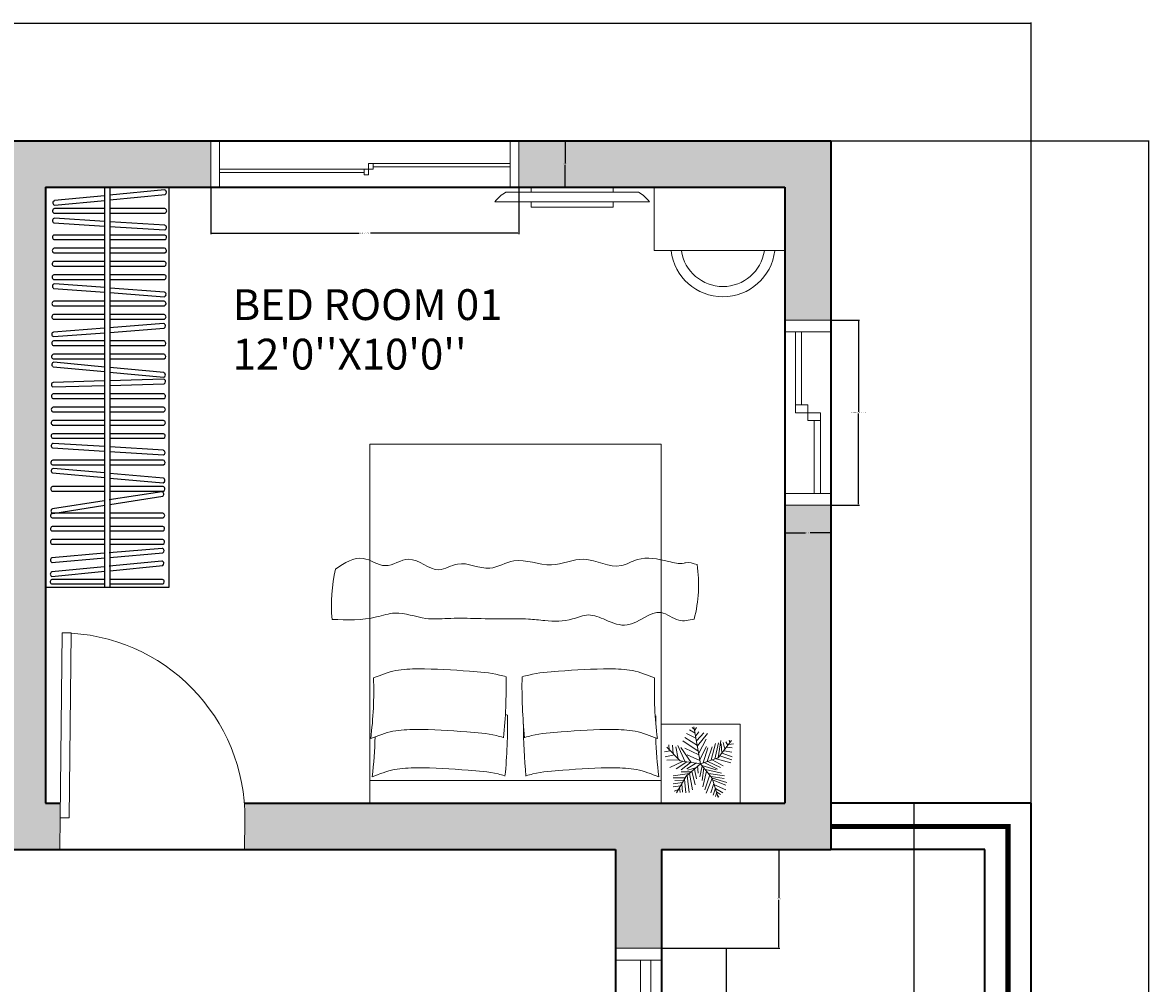
# Model space of a CAD drawing. Units: inches. Extents: x 1789 to 2841, y 3180 to 3702.
# Tile 14 of 14: x 2606 to 2825, y 3491 to 3678. Entities that reach past the tile are written whole.
import ezdxf

# ---------------------------------------------------------------- set-up
doc = ezdxf.new("R2010")
doc.units = ezdxf.units.IN
doc.header["$MEASUREMENT"] = 0
for name, color, linetype, lineweight in [('A-ANNO-DIMS', 2, 'Continuous', 18), ('A-AREA-IDEN', 7, 'Continuous', 18), ('A-EQPM', 8, 'Continuous', 18), ('A-FLOR-CASE', 34, 'Continuous', 25), ('A-FLOR-HRAL', 40, 'Continuous', 18), ('A-WALL', 40, 'Continuous', 35), ('A-WALL-PATT', 252, 'Continuous', 13), ('DORS', 70, 'Continuous', 18), ('FURNITURE', 34, 'Continuous', 18), ('WINDOWS', 130, 'Continuous', 18)]:
    doc.layers.add(name, color=color, linetype=linetype, lineweight=lineweight)
doc.styles.get("Standard").update_dxf_attribs({"font": 'arial.ttf'})
doc.dimstyles.get("Standard").update_dxf_attribs({"dimtxt": 0.18, "dimasz": 0.18, "dimexe": 0.18, "dimexo": 0.0625, "dimgap": 0.09, "dimtad": 0, "dimtih": 1, "dimtoh": 1, "dimdec": 0, "dimzin": 0, "dimdsep": 46, "dimlunit": 3, "dimtxsty": 'Standard', "dimcen": 0.09, "dimadec": 0, "dimazin": 0, "dimtfac": 1, "dimtdec": 0, "dimtofl": 0, "dimtmove": 0, "dimatfit": 3, "dimfxl": 1, "dimtolj": 1, "dimtzin": 0, "dimarcsym": 0})

# ---------------------------------------------------------------- blocks, each defined once
blk = doc.blocks.new('HYJ')
for p, q in [((2206.12, 3649.67), (2234.3, 3649.67)), ((2206.12, 3649), (2234.3, 3649)), ((2236.02, 3650.77), (2262.74, 3650.77)), ((2236.02, 3650.11), (2262.74, 3650.11))]:
    blk.add_line(p, q)
for points in [[(2204.43, 3646.16), (2264.43, 3646.16), (2264.43, 3655.16), (2204.43, 3655.16)], [(2204.43, 3655.16), (2206.12, 3655.16), (2206.12, 3646.16), (2204.43, 3646.16)], [(2264.43, 3655.16), (2262.74, 3655.16), (2262.74, 3646.16), (2264.43, 3646.16)], [(2234.3, 3649.67), (2235.16, 3649.67), (2235.16, 3648.56), (2234.3, 3648.56)], [(2235.16, 3650.77), (2236.02, 3650.77), (2236.02, 3649.67), (2235.16, 3649.67)]]:
    blk.add_lwpolyline(points, close=True)
blk = doc.blocks.new('KIK')
for p, q in [((2336.3, 3607.04), (2336.3, 3621.23)), ((2337.52, 3607.04), (2337.52, 3621.23)), ((2339.95, 3603.98), (2339.95, 3589.79)), ((2341.17, 3603.98), (2341.17, 3589.79))]:
    blk.add_line(p, q)
for points in [[(2343.23, 3623.51), (2343.23, 3587.51), (2334.23, 3587.51), (2334.23, 3623.51)], [(2343.23, 3623.51), (2334.23, 3623.51), (2334.23, 3621.23), (2343.23, 3621.23)], [(2338.73, 3605.51), (2336.3, 3605.51), (2336.3, 3607.04), (2338.73, 3607.04)], [(2341.17, 3603.98), (2338.73, 3603.98), (2338.73, 3605.51), (2341.17, 3605.51)], [(2343.23, 3587.51), (2334.23, 3587.51), (2334.23, 3589.79), (2343.23, 3589.79)]]:
    blk.add_lwpolyline(points, close=True)
blk = doc.blocks.new('CUBOARD')
for p, q in [((2183.73, 3646.16), (2183.73, 3568.16)), ((2184.71, 3646.16), (2184.71, 3568.16))]:
    blk.add_line(p, q)
blk.add_lwpolyline([(2172.23, 3646.16), (2196.23, 3646.16), (2196.23, 3568.16), (2172.23, 3568.16)], close=True)
for points in [[(2195.39, 3645.6), (2184.67, 3644.55)], [(2184.76, 3643.66), (2195.54, 3644.71)], [(2195.78, 3645.16), (2195.78, 3645.18)], [(2183.69, 3644.46), (2173.95, 3643.51)], [(2173.97, 3642.61), (2183.78, 3643.57)], [(2173.86, 3641.08), (2183.73, 3641.08)], [(2183.73, 3641.98), (2173.93, 3641.98)], [(2195.47, 3641.98), (2184.71, 3641.98)], [(2184.71, 3641.08), (2195.53, 3641.08)], [(2195.82, 3641.5), (2195.82, 3641.53)], [(2173.84, 3639.19), (2183.7, 3638.57)], [(2183.76, 3639.46), (2173.96, 3640.08)], [(2184.68, 3638.5), (2195.46, 3637.81)], [(2195.45, 3638.71), (2184.74, 3639.4)], [(2195.77, 3638.22), (2195.78, 3638.24)], [(2173.83, 3635.92), (2183.73, 3635.92)], [(2183.73, 3636.82), (2173.9, 3636.82)], [(2195.43, 3636.82), (2184.71, 3636.82)], [(2184.71, 3635.92), (2195.5, 3635.92)], [(2195.78, 3636.35), (2195.78, 3636.37)], [(2183.73, 3634.24), (2173.88, 3634.24)], [(2195.42, 3634.24), (2184.71, 3634.24)], [(2195.77, 3633.77), (2195.77, 3633.79)], [(2173.81, 3633.34), (2183.73, 3633.34)], [(2183.73, 3631.66), (2173.86, 3631.66)], [(2184.71, 3633.34), (2195.48, 3633.34)], [(2195.4, 3631.66), (2184.71, 3631.66)], [(2173.8, 3630.76), (2183.73, 3630.76)], [(2184.71, 3630.76), (2195.47, 3630.76)], [(2195.75, 3631.19), (2195.75, 3631.21)], [(2173.78, 3628.19), (2183.73, 3628.19)], [(2183.73, 3629.08), (2173.85, 3629.08)], [(2183.8, 3626.57), (2173.93, 3627.31)], [(2195.38, 3629.08), (2184.71, 3629.08)], [(2184.71, 3628.19), (2195.45, 3628.19)], [(2195.73, 3628.61), (2195.73, 3628.63)], [(2173.79, 3626.43), (2183.74, 3625.68)], [(2184.71, 3625.61), (2195.4, 3624.81)], [(2195.4, 3625.7), (2184.78, 3626.5)], [(2195.72, 3625.21), (2195.72, 3625.23)], [(2173.75, 3623.03), (2183.73, 3623.03)], [(2183.73, 3623.92), (2173.81, 3623.92)], [(2195.35, 3623.92), (2184.71, 3623.92)], [(2184.71, 3623.03), (2195.42, 3623.03)], [(2195.7, 3623.45), (2195.7, 3623.48)], [(2183.73, 3621.34), (2173.8, 3621.34)], [(2195.33, 3621.34), (2184.71, 3621.34)], [(2195.68, 3620.87), (2195.68, 3620.9)], [(2173.73, 3620.45), (2183.73, 3620.45)], [(2183.67, 3618.69), (2173.75, 3617.93)], [(2195.22, 3619.57), (2184.65, 3618.76)], [(2184.71, 3620.45), (2195.4, 3620.45)], [(2184.71, 3617.87), (2195.35, 3618.68)], [(2195.6, 3619.13), (2195.6, 3619.15)], [(2173.75, 3617.03), (2183.74, 3617.8)], [(2183.73, 3616.19), (2173.77, 3616.19)], [(2195.3, 3616.19), (2184.71, 3616.19)], [(2173.7, 3615.29), (2183.73, 3615.29)], [(2184.71, 3615.29), (2195.37, 3615.29)], [(2195.65, 3615.71), (2195.65, 3615.74)], [(2173.68, 3612.71), (2183.73, 3612.71)], [(2183.73, 3613.61), (2173.75, 3613.61)], [(2183.78, 3611.12), (2173.82, 3612.07)], [(2195.28, 3613.61), (2184.71, 3613.61)], [(2184.71, 3612.71), (2195.35, 3612.71)], [(2195.63, 3613.14), (2195.63, 3613.16)], [(2173.67, 3611.18), (2183.69, 3610.23)], [(2184.67, 3610.14), (2195.24, 3609.13)], [(2195.26, 3610.03), (2184.75, 3611.03)], [(2195.56, 3609.53), (2195.57, 3609.55)], [(2173.66, 3607.23), (2183.75, 3607.53)], [(2183.72, 3608.42), (2173.71, 3608.13)], [(2195.23, 3608.76), (2184.7, 3608.45)], [(2184.73, 3607.55), (2195.33, 3607.87)], [(2195.6, 3608.3), (2195.6, 3608.32)], [(2183.73, 3605.87), (2173.7, 3605.87)], [(2195.23, 3605.87), (2184.71, 3605.87)], [(2195.58, 3605.4), (2195.58, 3605.42)], [(2173.63, 3604.98), (2183.73, 3604.98)], [(2183.73, 3603.29), (2173.68, 3603.29)], [(2184.71, 3604.98), (2195.3, 3604.98)], [(2195.22, 3603.29), (2184.71, 3603.29)], [(2173.61, 3602.4), (2183.73, 3602.4)], [(2183.73, 3600.71), (2173.67, 3600.71)], [(2184.71, 3602.4), (2195.28, 3602.4)], [(2195.2, 3600.71), (2184.71, 3600.71)], [(2195.57, 3602.82), (2195.57, 3602.84)], [(2173.6, 3599.82), (2183.73, 3599.82)], [(2184.71, 3599.82), (2195.27, 3599.82)], [(2195.55, 3600.24), (2195.55, 3600.27)], [(2173.58, 3597.24), (2183.73, 3597.24)], [(2183.73, 3598.13), (2173.65, 3598.13)], [(2195.18, 3598.13), (2184.71, 3598.13)], [(2184.71, 3597.24), (2195.25, 3597.24)], [(2195.53, 3597.66), (2195.53, 3597.69)], [(2173.56, 3595.36), (2183.71, 3594.72)], [(2183.77, 3595.62), (2173.68, 3596.25)], [(2184.69, 3594.66), (2195.19, 3594)], [(2195.18, 3594.9), (2184.74, 3595.55)], [(2195.5, 3594.4), (2195.5, 3594.43)], [(2173.55, 3592.08), (2183.73, 3592.08)], [(2183.73, 3592.98), (2173.62, 3592.98)], [(2195.15, 3592.98), (2184.71, 3592.98)], [(2184.71, 3592.08), (2195.22, 3592.08)], [(2195.5, 3592.5), (2195.5, 3592.53)], [(2173.57, 3590.49), (2183.74, 3589.59)], [(2183.73, 3590.49), (2173.72, 3591.37)], [(2195.17, 3589.47), (2184.71, 3590.4)], [(2183.73, 3587.82), (2173.58, 3587.82)], [(2184.71, 3589.5), (2195.16, 3588.58)], [(2195.12, 3587.82), (2184.71, 3587.82)], [(2195.48, 3588.97), (2195.48, 3589)], [(2173.51, 3586.92), (2183.73, 3586.92)], [(2194.84, 3586.83), (2184.58, 3585.23)], [(2184.71, 3586.92), (2195.19, 3586.92)], [(2184.71, 3584.34), (2195.04, 3585.95)], [(2195.26, 3586.41), (2195.25, 3586.44)], [(2195.47, 3587.35), (2195.47, 3587.37)], [(2183.61, 3585.08), (2173.56, 3583.51)], [(2173.63, 3582.62), (2183.75, 3584.19)], [(2173.48, 3581.77), (2183.73, 3581.77)], [(2183.73, 3582.66), (2173.55, 3582.66)], [(2195.08, 3582.66), (2184.71, 3582.66)], [(2184.71, 3581.77), (2195.15, 3581.77)], [(2195.43, 3582.19), (2195.43, 3582.21)], [(2173.46, 3579.19), (2183.73, 3579.19)], [(2183.73, 3580.08), (2173.53, 3580.08)], [(2195.07, 3580.08), (2184.71, 3580.08)], [(2184.71, 3579.19), (2195.14, 3579.19)], [(2195.42, 3579.61), (2195.42, 3579.63)], [(2173.45, 3576.61), (2183.73, 3576.61)], [(2183.73, 3577.5), (2173.52, 3577.5)], [(2195.05, 3577.5), (2184.71, 3577.5)], [(2184.71, 3576.61), (2195.12, 3576.61)], [(2195.4, 3577.03), (2195.4, 3577.05)], [(2183.66, 3574.84), (2173.46, 3573.95)], [(2194.92, 3575.81), (2184.64, 3574.92)], [(2184.71, 3574.03), (2195.06, 3574.93)], [(2195.31, 3575.37), (2195.31, 3575.4)], [(2183.65, 3572.24), (2173.45, 3571.25)], [(2173.47, 3573.05), (2183.74, 3573.94)], [(2194.88, 3573.34), (2184.63, 3572.34)], [(2184.71, 3571.45), (2195.04, 3572.46)], [(2195.28, 3572.91), (2195.27, 3572.93)], [(2173.47, 3570.35), (2183.74, 3571.35)], [(2173.4, 3568.87), (2183.73, 3568.87)], [(2183.73, 3569.77), (2173.47, 3569.77)], [(2195, 3569.77), (2184.71, 3569.77)], [(2184.71, 3568.87), (2195.07, 3568.87)], [(2195.35, 3569.29), (2195.35, 3569.32)]]:
    blk.add_lwpolyline(points)
for centre, start, end in [((2195.31, 3645.13), 7.0195, 80.386), ((2195.31, 3645.13), 299.464, 4.1032), ((2174.12, 3643.06), 110.7367, 251.6587), ((2174.06, 3641.52), 105.1753, 246.0974), ((2195.34, 3641.52), 1.4582, 74.8247), ((2195.34, 3641.52), 293.9026, 358.5418), ((2174.06, 3639.62), 101.5232, 242.4452), ((2195.3, 3638.26), 357.8061, 71.1726), ((2195.3, 3638.26), 290.2505, 354.8897), ((2174.02, 3636.36), 105.1753, 246.0974), ((2195.31, 3636.36), 1.4582, 74.8247), ((2195.31, 3636.36), 293.9026, 358.5418), ((2174.01, 3633.78), 105.1753, 246.0974), ((2195.29, 3633.78), 1.4582, 74.8247), ((2195.29, 3633.78), 293.9026, 358.5418), ((2173.99, 3631.2), 105.1753, 246.0974), ((2195.27, 3631.2), 1.4582, 74.8247), ((2195.27, 3631.2), 293.9026, 358.5418), ((2173.97, 3628.62), 105.1753, 246.0974), ((2174.02, 3626.85), 100.888, 241.81), ((2195.26, 3628.62), 1.4582, 74.8247), ((2195.26, 3628.62), 293.9026, 358.5418), ((2195.24, 3625.25), 357.1709, 70.5374), ((2195.24, 3625.25), 289.6153, 354.2545), ((2173.94, 3623.46), 105.1753, 246.0974), ((2195.22, 3623.46), 1.4582, 74.8247), ((2195.22, 3623.46), 293.9026, 358.5418), ((2173.92, 3620.88), 105.1753, 246.0974), ((2195.21, 3620.88), 1.4582, 74.8247), ((2195.21, 3620.88), 293.9026, 358.5418), ((2195.13, 3619.1), 5.8369, 79.2034), ((2195.13, 3619.1), 298.2814, 2.9206), ((2173.89, 3615.73), 105.1753, 246.0974), ((2173.9, 3617.48), 109.5541, 250.4761), ((2195.17, 3615.73), 1.4582, 74.8247), ((2195.17, 3615.73), 293.9026, 358.5418), ((2173.87, 3613.15), 105.1753, 246.0974), ((2173.9, 3611.6), 99.7479, 240.6699), ((2195.16, 3613.15), 1.4582, 74.8247), ((2195.16, 3613.15), 293.9026, 358.5418), ((2195.09, 3609.58), 288.4752, 353.1144), ((2195.09, 3609.58), 356.0307, 69.3973), ((2173.84, 3607.67), 106.858, 247.78), ((2195.12, 3608.3), 3.1408, 76.5073), ((2195.12, 3608.3), 295.5853, 0.2245), ((2173.82, 3605.41), 105.1753, 246.0974), ((2195.11, 3605.41), 1.4582, 74.8247), ((2195.11, 3605.41), 293.9026, 358.5418), ((2173.81, 3602.83), 105.1753, 246.0974), ((2195.09, 3602.83), 1.4582, 74.8247), ((2173.79, 3600.25), 105.1753, 246.0974), ((2195.08, 3600.25), 1.4582, 74.8247), ((2195.09, 3602.83), 293.9026, 358.5418), ((2195.08, 3600.25), 293.9026, 358.5418), ((2173.77, 3597.67), 105.1753, 246.0974), ((2195.06, 3597.67), 1.4582, 74.8247), ((2195.06, 3597.67), 293.9026, 358.5418), ((2173.78, 3595.78), 101.566, 242.4881), ((2195.02, 3594.44), 357.8489, 71.2154), ((2195.02, 3594.44), 290.2933, 354.9325), ((2173.74, 3592.52), 105.1753, 246.0974), ((2195.03, 3592.52), 1.4582, 74.8247), ((2195.03, 3592.52), 293.9026, 358.5418), ((2173.8, 3590.9), 100.1162, 241.0382), ((2173.71, 3587.36), 105.1753, 246.0974), ((2194.99, 3587.36), 1.4582, 74.8247), ((2195.01, 3589.03), 288.8435, 353.4827), ((2195.01, 3589.03), 356.399, 69.7655), ((2194.79, 3586.35), 10.3063, 83.6728), ((2194.79, 3586.35), 302.7507, 7.3899), ((2194.99, 3587.36), 293.9026, 358.5418), ((2173.75, 3583.08), 114.0234, 254.9455), ((2173.67, 3582.2), 105.1753, 246.0974), ((2194.96, 3582.2), 1.4582, 74.8247), ((2194.96, 3582.2), 293.9026, 358.5418), ((2173.66, 3579.62), 105.1753, 246.0974), ((2194.94, 3579.62), 1.4582, 74.8247), ((2194.94, 3579.62), 293.9026, 358.5418), ((2173.64, 3577.04), 105.1753, 246.0974), ((2194.93, 3577.04), 1.4582, 74.8247), ((2194.93, 3577.04), 293.9026, 358.5418), ((2194.83, 3575.34), 6.4142, 79.7807), ((2194.83, 3575.34), 298.8587, 3.4979), ((2173.63, 3573.5), 110.1314, 251.0534), ((2194.8, 3572.87), 7.0476, 80.4142), ((2194.8, 3572.87), 299.4921, 4.1313), ((2173.62, 3570.8), 110.7648, 251.6868), ((2173.59, 3569.31), 105.1753, 246.0974), ((2194.88, 3569.31), 1.4582, 74.8247), ((2194.88, 3569.31), 293.9026, 358.5418)]:
    blk.add_arc(centre, 0.476, start, end)
blk = doc.blocks.new('*U9')
for p, q in [((0, 0), (0, -6)), ((36, 0), (36, -6))]:
    blk.add_line(p, q)
blk.add_lwpolyline([(0, 0), (0, 36), (1.75, 36), (1.75, 0)], close=True)
blk.add_arc((0, 0), 36, 0, 90)
blk = doc.blocks.new('GTGTG')
for points in [[(2261.92, 3645.14), (2287.72, 3645.14)], [(2289.9, 3643.29), (2259.74, 3643.29)]]:
    blk.add_lwpolyline(points)
for points in [[(2266.82, 3646.16), (2282.82, 3646.16), (2282.82, 3645.14), (2266.82, 3645.14)], [(2266.82, 3643.29), (2282.82, 3643.29), (2282.82, 3642.27), (2266.82, 3642.27)]]:
    blk.add_lwpolyline(points, close=True)
for centre, start, end in [((2265.21, 3639.05), 118.4184, 142.2436), ((2284.43, 3639.05), 37.7564, 61.5816)]:
    blk.add_arc(centre, 6.92, start, end)
blk = doc.blocks.new('WINDOW')
for p, q in [((1997.14, 3495.61), (1997.14, 3458.2)), ((1999.14, 3495.61), (1999.14, 3458.2)), ((1995.14, 3457.08), (1995.14, 3416.32)), ((1997.14, 3457.08), (1997.14, 3416.32))]:
    blk.add_line(p, q)
for points in [[(1992.23, 3497.95), (2001.23, 3497.95), (2001.23, 3413.99), (1992.23, 3413.99)], [(1992.23, 3497.95), (2001.23, 3497.95), (2001.23, 3495.61), (1992.23, 3495.61)], [(1997.14, 3457.08), (1999.14, 3457.08), (1999.14, 3458.2), (1997.14, 3458.2)], [(1995.14, 3455.97), (1997.14, 3455.97), (1997.14, 3457.08), (1995.14, 3457.08)], [(1992.23, 3413.99), (2001.23, 3413.99), (2001.23, 3416.32), (1992.23, 3416.32)]]:
    blk.add_lwpolyline(points, close=True)
blk = doc.blocks.new('*U22')
for p, q in [((-8.737, 47.138), (-17.069, 52.711)), ((-10.186, 53.64), (-13.084, 55.962)), ((0, 0), (-10.5, 57)), ((-9.099, 51.782), (-6.563, 55.962)), ((-3.665, 19.273), (-27.574, 35.527)), ((-5.114, 28.097), (-24.676, 40.636)), ((-7.288, 39.707), (-21.778, 46.673)), ((-7.65, 43.423), (-2.578, 49.46)), ((-5.839, 35.992), (4.667, 48.067)), ((-5.114, 27.632), (10.463, 46.673)), ((-2.941, 16.486), (8.652, 37.85)), ((27, 9), (48, 36)), ((27.127, 9.056), (31.112, 35.992)), ((44.153, 36.456), (45.239, 32.741)), ((-47.498, 19.737), (-55.83, 18.344)), ((-31.5, 4.5), (-52.5, 25.5)), ((-48.585, 21.131), (-49.309, 29.026)), ((-43.513, 28.561), (-42.427, 15.558)), ((-38.442, 26.239), (-34.819, 7.663)), ((-35.544, 28.097), (-24.314, 3.947)), ((-14.533, 2.09), (-30.834, 25.31)), ((-24.314, 23.917), (-2.941, 13.7)), ((-1.129, 6.734), (9.014, 26.704)), ((3.942, 1.625), (11.187, 24.381)), ((10.101, 3.483), (17.708, 26.239)), ((16.259, 5.805), (23.142, 31.348)), ((22.055, 7.198), (27.489, 32.277)), ((31.836, 30.883), (32.561, 16.486)), ((35.096, 32.741), (37.27, 22.524)), ((36.183, 19.737), (48.137, 17.88)), ((38.719, 34.134), (41.979, 28.561)), ((40.53, 25.775), (48.862, 24.846)), ((43.791, 29.954), (51.036, 30.883)), ((-40.615, 13.7), (-55.105, 10.913)), ((-33.37, 6.269), (-52.207, 5.34)), ((-28.299, 3.483), (-47.86, -5.805)), ((-21.416, 3.018), (-38.079, -8.128)), ((0, 0), (-31.5, 4.5)), ((-15.982, 2.09), (-30.11, -9.521)), ((0, 0), (-22.5, -19.5)), ((-6.563, 1.161), (-21.416, -8.128)), ((-20.691, 13.7), (-1.129, 4.876)), ((0, 0), (27, 9)), ((0, 0), (18, -22.5)), ((6.478, 1.625), (26.04, -8.592)), ((11.187, 3.483), (30.749, -5.805)), ((18.07, 5.805), (35.096, -3.483)), ((24.229, 7.663), (46.688, 1.625)), ((29.662, 12.307), (48.137, 6.269)), ((33.285, 16.486), (48.862, 10.913)), ((-17.431, -15.094), (-42.789, -18.809)), ((-15.257, -12.772), (-30.11, -12.772)), ((-6.563, -5.805), (-19.967, -9.985)), ((-17.069, -15.094), (-12.721, -40.172)), ((-13.446, -11.378), (-8.737, -32.741)), ((-9.461, -8.592), (-6.201, -23.453)), ((-4.752, -3.483), (-3.665, -14.629)), ((2.493, -3.019), (-1.491, -20.202)), ((1.769, -2.555), (24.229, -9.521)), ((5.029, -6.27), (2.131, -25.775)), ((9.014, -11.378), (3.58, -35.992)), ((14.085, -16.951), (6.478, -40.172)), ((7.565, -9.056), (32.198, -14.629)), ((12.274, -15.094), (36.907, -18.809)), ((-28.299, -29.026), (-42.789, -31.348)), ((-24.314, -21.596), (-42.427, -22.06)), ((-30.834, -34.135), (-42.427, -35.528)), ((-26.849, -26.24), (-40.253, -25.775)), ((-22.5, -19.5), (-37.5, -45)), ((-29.023, -30.884), (-27.936, -43.887)), ((-25.038, -23.918), (-22.865, -45.281)), ((-20.691, -18.345), (-17.793, -44.352)), ((18.07, -22.524), (8.289, -45.745)), ((20.244, -30.419), (15.897, -44.816)), ((16.259, -19.738), (36.183, -22.989)), ((18, -22.5), (27, -52.5)), ((18.433, -22.524), (40.53, -29.026)), ((19.157, -25.311), (38.719, -33.206)), ((21.331, -32.741), (39.081, -40.636)), ((-34.457, -39.708), (-40.978, -42.494)), ((-32.646, -36.921), (-31.921, -44.352)), ((22.78, -37.85), (19.519, -48.532)), ((22.78, -38.314), (34.372, -44.816)), ((24.591, -45.745), (23.142, -50.854)), ((24.591, -43.423), (30.749, -47.603)), ((26.764, -49.925), (28.213, -50.854))]:
    blk.add_line(p, q)
blk = doc.blocks.new('BEDD')
for points in [[(2235.4, 3526.16), (2292.14, 3526.16), (2292.14, 3596.12), (2235.4, 3596.12)], [(2292.14, 3526.16), (2307.57, 3526.16), (2307.57, 3541.59), (2292.14, 3541.59)], [(2235.4, 3526.16), (2292.14, 3526.16), (2292.14, 3530.61), (2235.4, 3530.61)]]:
    blk.add_lwpolyline(points, close=True)
for centre, radius, start, end in [((2273.81, 3568.71), 25.64, 344.9042, 8.8372), ((2259.99, 3564.78), 32.07, 167.4063, 185.0216), ((2163.47, 3548.06), 72.69, 352.674, 2.0029), ((2165.57, 3548.81), 96.38, 354.1175, 1.1854), ((2361.42, 3548.81), 96.38, 178.8146, 185.8825), ((2363.52, 3548.06), 72.69, 177.9971, 187.326), ((2165.85, 3541.35), 96.38, 354.1175, 1.1854), ((2361.69, 3541.35), 96.38, 179.877, 185.8825), ((2363.79, 3540.6), 72.69, 177.9971, 179.1531), ((2163.75, 3540.6), 72.69, 352.674, 358.8312), ((2363.79, 3540.6), 72.69, 181.3344, 187.326)]:
    blk.add_arc(centre, radius, start, end)
for points, knots in [([(2228.7, 3571.77), (2230.5, 3572.97), (2233.69, 3575.11), (2238.44, 3571.24), (2243.48, 3575.3), (2248.08, 3570.3), (2253.24, 3573.93), (2258.37, 3570.76), (2264.15, 3574.63), (2270.52, 3571.37), (2277.36, 3575.01), (2283.2, 3571.25), (2288.29, 3574.45), (2292.59, 3573.51), (2295.73, 3572.7), (2297.56, 3573.17), (2298.4, 3572.89), (2299.15, 3572.65)], [0, 0, 0, 0, 5.813057, 10.291797, 15.071674, 21.264477, 25.062958, 31.395117, 36.284741, 43.6566, 50.0956, 57.47363, 60.824937, 66.871309, 69.965772, 70.260383, 72.512122, 72.512122, 72.512122, 72.512122]), ([(2228.05, 3561.97), (2230.96, 3561.87), (2235.09, 3561.73), (2241.08, 3563.86), (2245.67, 3561.8), (2250.85, 3562.25), (2255.91, 3562.17), (2261.15, 3562), (2265.78, 3562.19), (2270.21, 3561.59), (2274.18, 3561.57), (2278.08, 3563.31), (2281.58, 3561.74), (2286.46, 3559.73), (2291.21, 3564.99), (2295.28, 3561.31), (2297.57, 3561.81), (2298.57, 3562.03)], [0, 0, 0, 0, 8.669632, 12.310458, 18.461416, 22.693385, 27.790985, 33.658819, 38.43562, 41.630677, 47.052462, 50.224855, 53.725722, 58.058029, 65.069701, 68.862462, 71.815525, 71.815525, 71.815525, 71.815525]), ([(2236.12, 3550.6), (2237.54, 3551.15), (2240.34, 3552.23), (2246.72, 3552.46), (2253.43, 3551.99), (2259.2, 3551.57), (2261.51, 3550.92), (2261.93, 3550.8)], [0, 0, 0, 0, 4.544245, 8.926813, 18.957656, 24.819591, 26.148375, 26.148375, 26.148375, 26.148375]), ([(2290.87, 3550.6), (2289.45, 3551.15), (2286.65, 3552.23), (2280.27, 3552.46), (2273.56, 3551.99), (2267.8, 3551.57), (2265.49, 3550.92), (2265.06, 3550.8)], [0, 0, 0, 0, 4.544245, 8.926813, 18.957656, 24.819591, 26.148375, 26.148375, 26.148375, 26.148375]), ([(2235.57, 3538.79), (2236.99, 3539.34), (2239.79, 3540.42), (2246.18, 3540.65), (2252.88, 3540.18), (2258.65, 3539.76), (2260.96, 3539.11), (2261.38, 3538.99)], [0, 0, 0, 0, 4.544245, 8.926813, 18.957656, 24.819591, 26.148375, 26.148375, 26.148375, 26.148375]), ([(2291.42, 3538.79), (2290, 3539.34), (2287.2, 3540.42), (2280.82, 3540.65), (2274.11, 3540.18), (2268.34, 3539.76), (2266.03, 3539.11), (2265.61, 3538.99)], [0, 0, 0, 0, 4.544245, 8.926813, 18.957656, 24.819591, 26.148375, 26.148375, 26.148375, 26.148375]), ([(2235.84, 3531.33), (2237.27, 3531.88), (2240.06, 3532.96), (2246.45, 3533.19), (2253.15, 3532.71), (2258.92, 3532.3), (2261.23, 3531.65), (2261.66, 3531.53)], [0, 0, 0, 0, 4.544245, 8.926813, 18.957656, 24.819591, 26.148375, 26.148375, 26.148375, 26.148375]), ([(2291.69, 3531.33), (2290.27, 3531.88), (2287.47, 3532.96), (2281.09, 3533.19), (2274.39, 3532.71), (2268.62, 3532.3), (2266.31, 3531.65), (2265.88, 3531.53)], [0, 0, 0, 0, 4.544245, 8.926813, 18.957656, 24.819591, 26.148375, 26.148375, 26.148375, 26.148375])]:
    blk.add_open_spline(points, degree=3, knots=knots)
for points in [[(2261.81, 3543.46), (2261.94, 3543.42), (2262.07, 3543.38), (2262.21, 3543.34)], [(2291.15, 3543.14), (2291.09, 3543.16), (2291.04, 3543.18), (2290.99, 3543.2)]]:
    blk.add_open_spline(points, degree=3)
at = {"xscale": 0.1258179792922857, "yscale": 0.1258179792922857, "zscale": 0.1258179792922857}
blk.add_blockref('*U22', (2299.85, 3533.87), dxfattribs=at)
blk = doc.blocks.new('CHAIR-DESK-ROUND')
for radius, start, end in [(10.16, 186.7458, 353.2542), (8.16, 188.4094, 351.5906)]:
    blk.add_arc((10.09, 10.16), radius, start, end)
blk = doc.blocks.new('*D31')
at = {"layer": 'A-ANNO-DIMS', "color": 0, "lineweight": -2, "transparency": 16777216}
for p, q in [((2642.43, 3646.1), (2642.43, 3636.98)), ((2702.43, 3646.1), (2702.43, 3636.98)), ((2642.61, 3637.16), (2671.31, 3637.16)), ((2702.25, 3637.16), (2673.55, 3637.16))]:
    blk.add_line(p, q, dxfattribs=at)
at = {"layer": 'A-ANNO-DIMS', "color": 0, "transparency": 16777216}
for points in [[(2642.61, 3637.19), (2642.61, 3637.13), (2642.43, 3637.16)], [(2702.25, 3637.19), (2702.25, 3637.13), (2702.43, 3637.16)]]:
    blk.add_solid(points, dxfattribs=at)
at = {"layer": 'Defpoints', "color": 0, "transparency": 16777216}
for p in [(2642.43, 3646.16), (2702.43, 3646.16), (2702.43, 3637.16)]:
    blk.add_point(p, dxfattribs=at)
at = {"layer": 'A-ANNO-DIMS', "color": 0, "transparency": 16777216, "insert": (2672.43, 3637.16), "char_height": 0.18, "attachment_point": 5}
blk.add_mtext('\\A1;WINDOW 60 TYP.', dxfattribs=at)
blk = doc.blocks.new('*D32')
at = {"layer": 'A-ANNO-DIMS', "color": 0, "lineweight": -2, "transparency": 16777216}
for p, q in [((2702.5, 3655.16), (2711.61, 3655.16)), ((2711.43, 3654.98), (2711.43, 3650.84)), ((2711.43, 3646.34), (2711.43, 3650.48)), ((2702.5, 3646.16), (2711.61, 3646.16))]:
    blk.add_line(p, q, dxfattribs=at)
at = {"layer": 'A-ANNO-DIMS', "color": 0, "transparency": 16777216}
for points in [[(2711.4, 3654.98), (2711.46, 3654.98), (2711.43, 3655.16)], [(2711.4, 3646.34), (2711.46, 3646.34), (2711.43, 3646.16)]]:
    blk.add_solid(points, dxfattribs=at)
at = {"layer": 'Defpoints', "color": 0, "transparency": 16777216}
for p in [(2702.43, 3655.16), (2711.43, 3655.16), (2702.43, 3646.16)]:
    blk.add_point(p, dxfattribs=at)
at = {"layer": 'A-ANNO-DIMS', "color": 0, "transparency": 16777216, "insert": (2711.43, 3650.66), "char_height": 0.18, "attachment_point": 5}
blk.add_mtext('\\A1;9 TYP.', dxfattribs=at)
blk = doc.blocks.new('*D33')
at = {"layer": 'A-ANNO-DIMS', "color": 0, "lineweight": -2, "transparency": 16777216}
for p, q in [((2763.3, 3620.23), (2768.81, 3620.23)), ((2768.63, 3620.05), (2768.63, 3602.41)), ((2768.63, 3584.41), (2768.63, 3602.04)), ((2763.3, 3584.23), (2768.81, 3584.23))]:
    blk.add_line(p, q, dxfattribs=at)
at = {"layer": 'A-ANNO-DIMS', "color": 0, "transparency": 16777216}
for points in [[(2768.6, 3620.05), (2768.66, 3620.05), (2768.63, 3620.23)], [(2768.6, 3584.41), (2768.66, 3584.41), (2768.63, 3584.23)]]:
    blk.add_solid(points, dxfattribs=at)
at = {"layer": 'Defpoints', "color": 0, "transparency": 16777216}
for p in [(2763.23, 3620.23), (2768.63, 3620.23), (2763.23, 3584.23)]:
    blk.add_point(p, dxfattribs=at)
at = {"layer": 'A-ANNO-DIMS', "color": 0, "transparency": 16777216, "insert": (2768.63, 3602.23), "char_height": 0.18, "attachment_point": 5}
blk.add_mtext('\\A1;BEDROOM WINDOW 36 TYP.', dxfattribs=at)
blk = doc.blocks.new('*D34')
at = {"layer": 'A-ANNO-DIMS', "color": 0, "lineweight": -2, "transparency": 16777216}
for p, q in [((2754.23, 3584.17), (2754.23, 3578.65)), ((2763.23, 3584.17), (2763.23, 3578.65)), ((2754.41, 3578.83), (2758.28, 3578.83)), ((2763.05, 3578.83), (2759.19, 3578.83))]:
    blk.add_line(p, q, dxfattribs=at)
at = {"layer": 'A-ANNO-DIMS', "color": 0, "transparency": 16777216}
for points in [[(2754.41, 3578.86), (2754.41, 3578.8), (2754.23, 3578.83)], [(2763.05, 3578.86), (2763.05, 3578.8), (2763.23, 3578.83)]]:
    blk.add_solid(points, dxfattribs=at)
at = {"layer": 'Defpoints', "color": 0, "transparency": 16777216}
for p in [(2754.23, 3584.23), (2763.23, 3584.23), (2763.23, 3578.83)]:
    blk.add_point(p, dxfattribs=at)
at = {"layer": 'A-ANNO-DIMS', "color": 0, "transparency": 16777216, "insert": (2758.73, 3578.83), "char_height": 0.18, "attachment_point": 5}
blk.add_mtext('\\A1;9 TYP.', dxfattribs=at)
blk = doc.blocks.new('*D35')
at = {"layer": 'A-ANNO-DIMS', "color": 0, "lineweight": -2, "transparency": 16777216}
for p, q in [((2730.3, 3497.95), (2743.01, 3497.95)), ((2742.83, 3497.77), (2742.83, 3456.15)), ((2742.83, 3414.17), (2742.83, 3455.78)), ((2730.3, 3413.99), (2743.01, 3413.99))]:
    blk.add_line(p, q, dxfattribs=at)
at = {"layer": 'A-ANNO-DIMS', "color": 0, "transparency": 16777216}
for points in [[(2742.8, 3497.77), (2742.86, 3497.77), (2742.83, 3497.95)], [(2742.8, 3414.17), (2742.86, 3414.17), (2742.83, 3413.99)]]:
    blk.add_solid(points, dxfattribs=at)
at = {"layer": 'Defpoints', "color": 0, "transparency": 16777216}
for p in [(2730.23, 3497.95), (2742.83, 3497.95), (2730.23, 3413.99)]:
    blk.add_point(p, dxfattribs=at)
at = {"layer": 'A-ANNO-DIMS', "color": 0, "transparency": 16777216, "insert": (2742.83, 3455.97), "char_height": 0.18, "attachment_point": 5}
blk.add_mtext('\\A1;LIVING WINDOW 84 TYP.', dxfattribs=at)
blk = doc.blocks.new('*D95')
at = {"layer": 'A-ANNO-DIMS', "color": 0, "lineweight": -2, "transparency": 16777216}
for p, q in [((2397.23, 3655.22), (2397.23, 3678.19)), ((2397.41, 3678.01), (2599.44, 3678.01)), ((2802.05, 3678.01), (2600.03, 3678.01)), ((2802.23, 3526.22), (2802.23, 3678.19))]:
    blk.add_line(p, q, dxfattribs=at)
at = {"layer": 'A-ANNO-DIMS', "color": 0, "transparency": 16777216}
for points in [[(2397.41, 3678.04), (2397.41, 3677.98), (2397.23, 3678.01)], [(2802.05, 3678.04), (2802.05, 3677.98), (2802.23, 3678.01)]]:
    blk.add_solid(points, dxfattribs=at)
at = {"layer": 'Defpoints', "color": 0, "transparency": 16777216}
for p in [(2802.23, 3678.01), (2397.23, 3655.16), (2802.23, 3526.16)]:
    blk.add_point(p, dxfattribs=at)
at = {"layer": 'A-ANNO-DIMS', "color": 0, "transparency": 16777216, "insert": (2599.73, 3678.01), "char_height": 0.18, "attachment_point": 5}
blk.add_mtext('\\A1;405', dxfattribs=at)
blk = doc.blocks.new('*D96')
at = {"layer": 'A-ANNO-DIMS', "color": 0, "lineweight": -2, "transparency": 16777216}
for p, q in [((2763.3, 3655.16), (2825.26, 3655.16)), ((2825.08, 3654.98), (2825.08, 3429.34)), ((2825.08, 3203.34), (2825.08, 3428.98)), ((2763.3, 3203.16), (2825.26, 3203.16))]:
    blk.add_line(p, q, dxfattribs=at)
at = {"layer": 'A-ANNO-DIMS', "color": 0, "transparency": 16777216}
for points in [[(2825.05, 3654.98), (2825.11, 3654.98), (2825.08, 3655.16)], [(2825.05, 3203.34), (2825.11, 3203.34), (2825.08, 3203.16)]]:
    blk.add_solid(points, dxfattribs=at)
at = {"layer": 'Defpoints', "color": 0, "transparency": 16777216}
for p in [(2763.23, 3655.16), (2763.23, 3203.16), (2825.08, 3203.16)]:
    blk.add_point(p, dxfattribs=at)
at = {"layer": 'A-ANNO-DIMS', "color": 0, "transparency": 16777216, "insert": (2825.08, 3429.16), "char_height": 0.18, "attachment_point": 5}
blk.add_mtext('\\A1;452', dxfattribs=at)
blk = doc.blocks.new('*D113')
at = {"layer": 'A-ANNO-DIMS', "color": 0, "lineweight": -2, "transparency": 16777216}
for p, q in [((2730.3, 3517.16), (2753.26, 3517.16)), ((2753.08, 3516.98), (2753.08, 3507.74)), ((2753.08, 3498.13), (2753.08, 3507.37)), ((2730.3, 3497.95), (2753.26, 3497.95))]:
    blk.add_line(p, q, dxfattribs=at)
at = {"layer": 'A-ANNO-DIMS', "color": 0, "transparency": 16777216}
for points in [[(2753.05, 3516.98), (2753.11, 3516.98), (2753.08, 3517.16)], [(2753.05, 3498.13), (2753.11, 3498.13), (2753.08, 3497.95)]]:
    blk.add_solid(points, dxfattribs=at)
at = {"layer": 'Defpoints', "color": 0, "transparency": 16777216}
for p in [(2730.23, 3517.16), (2730.23, 3497.95), (2753.08, 3497.95)]:
    blk.add_point(p, dxfattribs=at)
at = {"layer": 'A-ANNO-DIMS', "color": 0, "transparency": 16777216, "insert": (2753.08, 3507.55), "char_height": 0.18, "attachment_point": 5}
blk.add_mtext('\\A1;19.214', dxfattribs=at)
blk = doc.blocks.new('*D114')
at = {"layer": 'A-ANNO-DIMS', "color": 0, "lineweight": -2, "transparency": 16777216}
for p, q in [((2802.17, 3526.16), (2779.2, 3526.16)), ((2779.38, 3525.98), (2779.38, 3472.58)), ((2779.38, 3418.81), (2779.38, 3472.21)), ((2802.17, 3418.63), (2779.2, 3418.63))]:
    blk.add_line(p, q, dxfattribs=at)
at = {"layer": 'A-ANNO-DIMS', "color": 0, "transparency": 16777216}
for points in [[(2779.35, 3525.98), (2779.41, 3525.98), (2779.38, 3526.16)], [(2779.35, 3418.81), (2779.41, 3418.81), (2779.38, 3418.63)]]:
    blk.add_solid(points, dxfattribs=at)
at = {"layer": 'Defpoints', "color": 0, "transparency": 16777216}
for p in [(2779.38, 3526.16), (2802.23, 3526.16), (2802.23, 3418.63)]:
    blk.add_point(p, dxfattribs=at)
at = {"layer": 'A-ANNO-DIMS', "color": 0, "transparency": 16777216, "insert": (2779.38, 3472.4), "char_height": 0.18, "attachment_point": 5}
blk.add_mtext('\\A1;107.53', dxfattribs=at)

msp = doc.modelspace()

# ---------------------------------------------------------------- hatches: boundary and pattern name
at = {"layer": 'A-WALL-PATT'}
h = msp.add_hatch(color=256, dxfattribs=at)
h.dxf.hatch_style = 1
h.paths.add_polyline_path([(2490.2333, 3655.1608), (2397.2333, 3655.1608), (2397.2333, 3622.3936), (2406.2333, 3622.3936), (2406.2333, 3646.1608), (2490.2333, 3646.1608)])
h.paths.add_polyline_path([(2642.4325, 3655.1608), (2555.6786, 3655.1608), (2555.6786, 3646.1608), (2601.2333, 3646.1608), (2601.2333, 3640.1475), (2601.2333, 3568.1608), (2597.2333, 3568.1608), (2597.2333, 3565.4274), (2601.2333, 3565.4274), (2601.2333, 3528.1608), (2601.2333, 3517.1608), (2612.9879, 3517.1608), (2613.0522, 3523.352), (2613.0813, 3526.1608), (2610.2333, 3526.1608), (2610.2333, 3646.1608), (2634.2333, 3646.1608), (2642.4325, 3646.1608)])
h.paths.add_polyline_path([(2523.2333, 3646.1608), (2531.6786, 3646.1608), (2531.6786, 3655.1608), (2514.2333, 3655.1608), (2514.2333, 3646.1608), (2514.2333, 3621.0865), (2514.2333, 3564.976, -0.02086055), (2517.2333, 3565.1012), (2523.2333, 3565.1012), (2523.2333, 3565.4274), (2567.2333, 3565.4274), (2567.2333, 3568.1608), (2523.2333, 3568.1608)])
h = msp.add_hatch(color=256, dxfattribs=at)
h.dxf.hatch_style = 1
h.paths.add_polyline_path([(2763.2333, 3655.1608), (2702.4325, 3655.1608), (2702.4325, 3646.1608), (2754.2333, 3646.1608), (2754.2333, 3633.8369), (2754.2333, 3620.2279), (2763.2333, 3620.2279)])
h = msp.add_hatch(color=256, dxfattribs=at)
h.dxf.hatch_style = 1
h.paths.add_polyline_path([(2763.2333, 3584.2279), (2754.2333, 3584.2279), (2754.2333, 3526.1608), (2648.9424, 3526.1608, -0.02212562), (2649.0502, 3522.9781), (2648.9898, 3517.1608), (2721.2333, 3517.1608), (2721.2333, 3497.9466), (2730.2333, 3497.9466), (2730.2333, 3517.1608), (2763.2333, 3517.1608)])

# ---------------------------------------------------------------- linework, layer by layer
at = {"layer": 'A-FLOR-HRAL', "const_width": 1}
msp.add_lwpolyline([(2763.2333, 3521.6608), (2797.7333, 3521.6608), (2797.7333, 3413.0793, -0.09351003), (2792.6951, 3386.3751, 0.04972233), (2763.2333, 3356.4636)], format="xyb", dxfattribs=at)
at = {"layer": 'A-WALL'}
for p, q in [((2397.2333, 3655.1608), (2763.2333, 3655.1608)), ((2763.2333, 3655.1608), (2763.2333, 3517.1608)), ((2610.2333, 3646.1608), (2610.2333, 3526.1608)), ((2610.2333, 3646.1608), (2754.2333, 3646.1608)), ((2754.2333, 3646.1608), (2754.2333, 3526.1608)), ((2610.2333, 3526.1608), (2613.0813, 3526.1608)), ((2648.9424, 3526.1608), (2754.2333, 3526.1608)), ((2802.2333, 3526.1608), (2763.2333, 3526.1608)), ((2802.2333, 3418.6331), (2802.2333, 3526.1608)), ((2601.2333, 3517.1608), (2721.2333, 3517.1608)), ((2721.2333, 3517.1608), (2721.2333, 3376.1608)), ((2730.2333, 3517.1608), (2730.2333, 3385.1608)), ((2730.2333, 3517.1608), (2763.2333, 3517.1608)), ((2793.2333, 3517.1608), (2763.2333, 3517.1608)), ((2793.2333, 3418.6846), (2793.2333, 3517.1608))]:
    msp.add_line(p, q, dxfattribs=at)
at = {"layer": 'FURNITURE'}
msp.add_lwpolyline([(2754.2333, 3646.1608), (2728.7859, 3646.1608), (2728.7859, 3633.8369), (2754.2333, 3633.8369)], close=True, dxfattribs=at)

# ---------------------------------------------------------------- block references
at = {"layer": 'A-EQPM'}
msp.add_blockref('GTGTG', (438, 0), dxfattribs=at)
at = {"layer": 'A-FLOR-CASE'}
msp.add_blockref('CUBOARD', (438, 0), dxfattribs=at)
at = {"layer": 'DORS', "rotation": 359.4048883422561}
msp.add_blockref('*U9', (2613.0522, 3523.352), dxfattribs=at)
at = {"layer": 'FURNITURE'}
for name, p in [('CHAIR-DESK-ROUND', (2732.097, 3624.79)), ('BEDD', (438, 0))]:
    msp.add_blockref(name, p, dxfattribs=at)
at = {"layer": 'WINDOWS'}
for name, p in [('HYJ', (438, 0)), ('KIK', (420, -3.2831)), ('WINDOW', (729, 0))]:
    msp.add_blockref(name, p, dxfattribs=at)

# ---------------------------------------------------------------- texts
at = {"layer": 'A-ANNO-DIMS'}
msp.add_text("12'0''X10'0''", height=6, dxfattribs=at).set_placement((2646.6596, 3610.628))
at = {"layer": 'A-AREA-IDEN'}
msp.add_text('BED ROOM 01', height=6, dxfattribs=at).set_placement((2646.6596, 3620.2665))

# ---------------------------------------------------------------- dimensions: what is measured, and where the dimension line sits
at = {"layer": 'A-ANNO-DIMS'}
dim = msp.add_linear_dim(base=(2802.2333, 3678.0108), p1=(2397.2333, 3655.1608), p2=(2802.2333, 3526.1608), dimstyle='Standard', override={"dimdec": 0, "dimlfac": 1, "dimrnd": 0, "dimzin": 0, "dimdsep": 46, "dimlunit": 2}, dxfattribs=at)
dim.commit()
dim.dimension.update_dxf_attribs({"geometry": '*D95', "text_midpoint": (2599.7333, 3678.0108)})
for base, p1, p2, text, picture, middle in [((2711.4325, 3655.1608), (2702.4325, 3646.1608), (2702.4325, 3655.1608), '<> TYP.', '*D32', (2711.4325, 3650.6608)), ((2768.6333, 3620.2279), (2763.2333, 3584.2279), (2763.2333, 3620.2279), 'BEDROOM WINDOW <> TYP.', '*D33', (2768.6333, 3602.2279)), ((2742.8271, 3497.9466), (2730.2333, 3413.9882), (2730.2333, 3497.9466), 'LIVING WINDOW <> TYP.', '*D35', (2742.8271, 3455.9674))]:
    dim = msp.add_linear_dim(base=base, p1=p1, p2=p2, angle=90, text=text, dimstyle='Standard', override={"dimdec": 0, "dimlfac": 1, "dimrnd": 0, "dimzin": 0, "dimdsep": 46, "dimlunit": 2}, dxfattribs=at)
    dim.commit()
    dim.dimension.update_dxf_attribs({"geometry": picture, "text_midpoint": middle})
for base, p1, p2, angle, override, picture, middle in [((2825.0833, 3203.1608), (2763.2333, 3655.1608), (2763.2333, 3203.1608), 90, {"dimdec": 0, "dimlfac": 1, "dimrnd": 0, "dimzin": 0, "dimdsep": 46, "dimlunit": 2}, '*D96', (2825.0833, 3429.1608)), ((2779.3833, 3526.1608), (2802.2333, 3418.6331), (2802.2333, 3526.1608), 90, {"dimdec": 2, "dimlfac": 1, "dimrnd": 0, "dimzin": 0, "dimdsep": 46, "dimlunit": 2}, '*D114', (2779.3833, 3472.3969)), ((2753.0833, 3497.9466), (2730.2333, 3517.1608), (2730.2333, 3497.9466), 270, {"dimdec": 3, "dimlfac": 1, "dimrnd": 0, "dimzin": 0, "dimdsep": 46, "dimlunit": 2}, '*D113', (2753.0833, 3507.5537))]:
    dim = msp.add_linear_dim(base=base, p1=p1, p2=p2, angle=angle, dimstyle='Standard', override=override, dxfattribs=at)
    dim.commit()
    dim.dimension.update_dxf_attribs({"geometry": picture, "text_midpoint": middle})
for base, p1, p2, text, picture, middle in [((2702.4325, 3637.1608), (2642.4325, 3646.1608), (2702.4325, 3646.1608), 'WINDOW <> TYP.', '*D31', (2672.4325, 3637.1608)), ((2763.2333, 3578.8279), (2754.2333, 3584.2279), (2763.2333, 3584.2279), '<> TYP.', '*D34', (2758.7333, 3578.8279))]:
    dim = msp.add_linear_dim(base=base, p1=p1, p2=p2, text=text, dimstyle='Standard', override={"dimdec": 0, "dimlfac": 1, "dimrnd": 0, "dimzin": 0, "dimdsep": 46, "dimlunit": 2}, dxfattribs=at)
    dim.commit()
    dim.dimension.update_dxf_attribs({"geometry": picture, "text_midpoint": middle})

doc.saveas('drawing.dxf')
